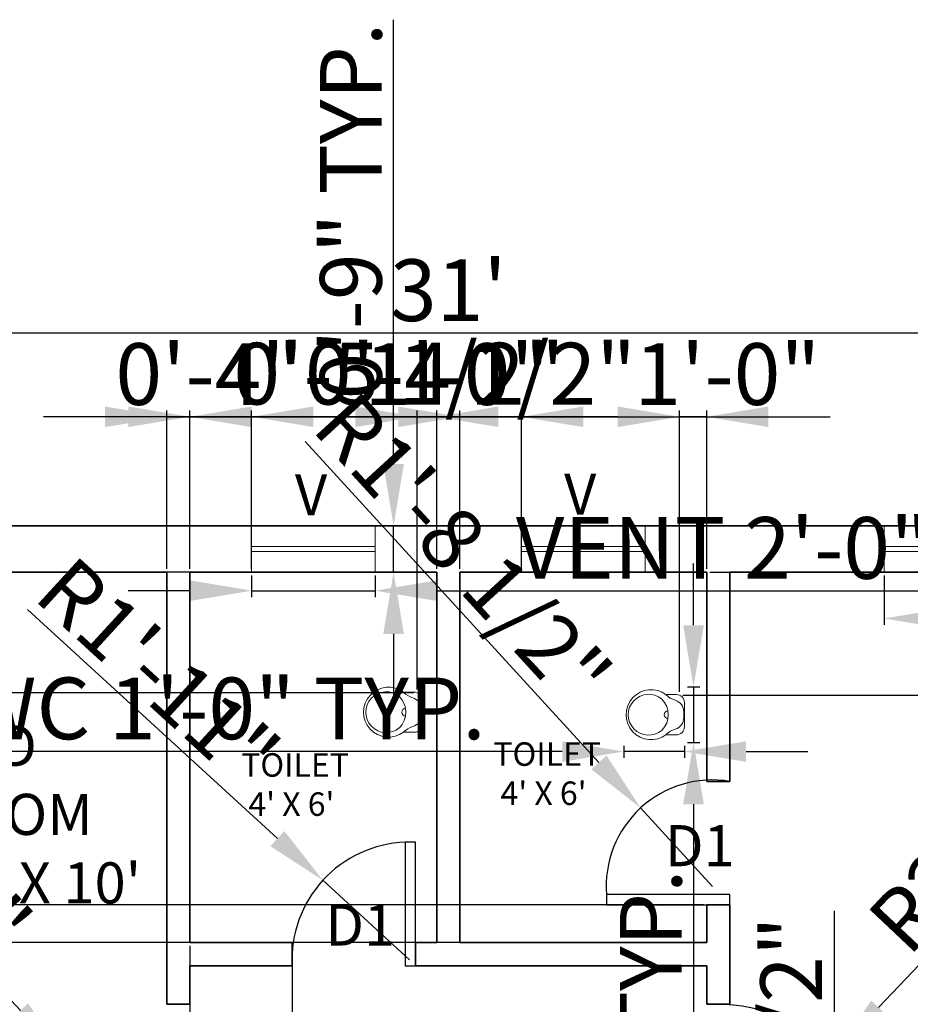
# Model space of a CAD drawing. Units: inches. Extents: x 2122 to 2726, y 1923 to 2370.
# Tile 4 of 6: x 2333 to 2506, y 2178 to 2370. Entities that reach past the tile are written whole.
import ezdxf

# ---------------------------------------------------------------- set-up
doc = ezdxf.new("R2010")
doc.units = ezdxf.units.IN
for name, color, linetype, lineweight in [('A-ANNO-DIMS', 2, 'Continuous', 18), ('A-ANNO-TEXT', 7, 'Continuous', 18), ('A-AREA-IDEN', 7, 'Continuous', 25), ('A-DOOR', 3, 'Continuous', 25), ('A-FLOR-FIXT', 9, 'Continuous', 18), ('A-GLAZ', 4, 'Continuous', 18), ('A-WALL', 7, 'Continuous', 35)]:
    doc.layers.add(name, color=color, linetype=linetype, lineweight=lineweight)
doc.styles.get("Standard").update_dxf_attribs({"font": 'arial.ttf'})
doc.dimstyles.new('ISO-25', dxfattribs={"dimtxt": 12, "dimasz": 12, "dimexe": 1.25, "dimexo": 0.625, "dimtad": 1, "dimlunit": 3, "dimtxsty": 'Standard', "dimcen": 2.5, "dimadec": 0, "dimazin": 0, "dimtfac": 1, "dimtmove": 0, "dimatfit": 3, "dimfxl": 1, "dimarcsym": 0})

# ---------------------------------------------------------------- blocks, each defined once
blk = doc.blocks.new('A$C6EF51710')
at = {"linetype": 'ByBlock'}
for p, q in [((0.0508, 0.2843), (0.1169, 0.2843)), ((0, 0.0811), (0, 0.2335)), ((0.0041, 0.1392), (0.0041, 0.1755)), ((0.1169, 0.0303), (0.0508, 0.0303))]:
    blk.add_line(p, q, dxfattribs=at)
for centre, radius, start, end in [((0.2107, 0.1573), 0.1576, 232.89836, 127.10164), ((0.0508, 0.2335), 0.0508, 90, 180), ((0.0168, 0.3818), 0.1397, 287.10464, 315), ((0.2413, 0.1573), 0.1397, 135, 225), ((0.2254, 0.1573), 0.1289, 230.00836, 129.99164), ((0.0803, 0.1755), 0.0762, 107.10464, 180), ((0.0803, 0.1392), 0.0762, 180, 252.89536), ((0.1016, 0.1573), 0.0254, 275.21591, 84.78409), ((0.0508, 0.0811), 0.0508, 180, 270), ((0.0168, -0.0672), 0.1397, 45, 72.89536)]:
    blk.add_arc(centre, radius, start, end, dxfattribs=at)
blk = doc.blocks.new('*D10')
at = {"layer": 'A-ANNO-DIMS', "color": 0, "lineweight": -2, "transparency": 16777216}
for p, q in [((2232.51, 2271.86), (2232.51, 2309.99)), ((2244.51, 2308.74), (2588.01, 2308.74)), ((2600.01, 2271.86), (2600.01, 2309.99))]:
    blk.add_line(p, q, dxfattribs=at)
at = {"layer": 'A-ANNO-DIMS', "color": 0, "transparency": 16777216}
for points in [[(2244.51, 2310.74), (2244.51, 2306.74), (2232.51, 2308.74)], [(2588.01, 2310.74), (2588.01, 2306.74), (2600.01, 2308.74)]]:
    blk.add_solid(points, dxfattribs=at)
at = {"layer": 'Defpoints', "color": 0, "transparency": 16777216}
for p in [(2600.01, 2308.74), (2232.51, 2271.24), (2600.01, 2271.24)]:
    blk.add_point(p, dxfattribs=at)
at = {"layer": 'A-ANNO-DIMS', "color": 0, "transparency": 16777216, "insert": (2416.26, 2315.49), "char_height": 12, "attachment_point": 5}
blk.add_mtext("31'", dxfattribs=at)
blk = doc.blocks.new('WIN-60IN')
for p, q in [((0, 0), (0, 9)), ((60, 0), (60, 9)), ((0, 5), (60, 5)), ((0, 4), (60, 4))]:
    blk.add_line(p, q)
blk = doc.blocks.new('VENT-24IN')
for p, q in [((0, 0), (0, 9)), ((24, 0), (24, 9)), ((0, 5), (24, 5)), ((0, 4), (24, 4))]:
    blk.add_line(p, q)
blk = doc.blocks.new('DOOR-LEAF-24IN')
for p, q in [((2, 24), (0, 24)), ((0, 24), (0, 0)), ((2, 0), (2, 24)), ((0, 0), (2, 0))]:
    blk.add_line(p, q)
blk = doc.blocks.new('*D16')
at = {"layer": 'A-ANNO-DIMS', "color": 0, "lineweight": -2, "transparency": 16777216}
for p, q in [((2501.01, 2261.61), (2501.01, 2251.99)), ((2561.01, 2261.61), (2561.01, 2251.99)), ((2513.01, 2253.24), (2549.01, 2253.24)), ((2561.01, 2253.24), (2726.11, 2253.24))]:
    blk.add_line(p, q, dxfattribs=at)
at = {"layer": 'A-ANNO-DIMS', "color": 0, "transparency": 16777216}
for points in [[(2513.01, 2255.24), (2513.01, 2251.24), (2501.01, 2253.24)], [(2549.01, 2255.24), (2549.01, 2251.24), (2561.01, 2253.24)]]:
    blk.add_solid(points, dxfattribs=at)
at = {"layer": 'Defpoints', "color": 0, "transparency": 16777216}
for p in [(2501.01, 2262.24), (2561.01, 2262.24), (2561.01, 2253.24)]:
    blk.add_point(p, dxfattribs=at)
at = {"layer": 'A-ANNO-DIMS', "color": 0, "transparency": 16777216, "insert": (2649.56, 2260.07), "char_height": 12, "attachment_point": 5}
blk.add_mtext('WINDOW 5\'-0" TYP.', dxfattribs=at)
blk = doc.blocks.new('*D20')
at = {"layer": 'A-ANNO-DIMS', "color": 0, "lineweight": -2, "transparency": 16777216}
for p, q in [((2378.01, 2261.61), (2378.01, 2257.39)), ((2402.01, 2261.61), (2402.01, 2257.39)), ((2366.01, 2258.64), (2354.01, 2258.64)), ((2378.01, 2258.64), (2402.01, 2258.64)), ((2414.01, 2258.64), (2550.39, 2258.64))]:
    blk.add_line(p, q, dxfattribs=at)
at = {"layer": 'A-ANNO-DIMS', "color": 0, "transparency": 16777216}
for points in [[(2366.01, 2260.64), (2366.01, 2256.64), (2378.01, 2258.64)], [(2414.01, 2260.64), (2414.01, 2256.64), (2402.01, 2258.64)]]:
    blk.add_solid(points, dxfattribs=at)
at = {"layer": 'Defpoints', "color": 0, "transparency": 16777216}
for p in [(2378.01, 2262.24), (2402.01, 2262.24), (2402.01, 2258.64)]:
    blk.add_point(p, dxfattribs=at)
at = {"layer": 'A-ANNO-DIMS', "color": 0, "transparency": 16777216, "insert": (2488.2, 2265.39), "char_height": 12, "attachment_point": 5}
blk.add_mtext('VENT 2\'-0" TYP.', dxfattribs=at)
blk = doc.blocks.new('*D21')
at = {"layer": 'A-ANNO-DIMS', "color": 0, "lineweight": -2, "transparency": 16777216}
for p, q in [((2405.61, 2283.24), (2405.61, 2369.63)), ((2402.63, 2271.24), (2406.86, 2271.24)), ((2405.61, 2262.24), (2405.61, 2271.24)), ((2402.63, 2262.24), (2406.86, 2262.24)), ((2405.61, 2250.24), (2405.61, 2238.24))]:
    blk.add_line(p, q, dxfattribs=at)
at = {"layer": 'A-ANNO-DIMS', "color": 0, "transparency": 16777216}
for points in [[(2403.61, 2283.24), (2407.61, 2283.24), (2405.61, 2271.24)], [(2403.61, 2250.24), (2407.61, 2250.24), (2405.61, 2262.24)]]:
    blk.add_solid(points, dxfattribs=at)
at = {"layer": 'Defpoints', "color": 0, "transparency": 16777216}
for p in [(2402.01, 2271.24), (2405.61, 2271.24), (2402.01, 2262.24)]:
    blk.add_point(p, dxfattribs=at)
at = {"layer": 'A-ANNO-DIMS', "color": 0, "transparency": 16777216, "insert": (2398.86, 2332.43), "char_height": 12, "attachment_point": 5, "rotation": 90}
blk.add_mtext('0\'-9" TYP.', dxfattribs=at)
blk = doc.blocks.new('*D22')
at = {"layer": 'A-ANNO-DIMS', "color": 0, "lineweight": -2, "transparency": 16777216}
for p, q in [((2330.01, 2149.64), (2142.68, 2149.64)), ((2330.01, 2144.86), (2330.01, 2150.89)), ((2354.01, 2149.64), (2342.01, 2149.64)), ((2366.01, 2144.86), (2366.01, 2150.89))]:
    blk.add_line(p, q, dxfattribs=at)
at = {"layer": 'A-ANNO-DIMS', "color": 0, "transparency": 16777216}
for points in [[(2342.01, 2151.64), (2342.01, 2147.64), (2330.01, 2149.64)], [(2354.01, 2151.64), (2354.01, 2147.64), (2366.01, 2149.64)]]:
    blk.add_solid(points, dxfattribs=at)
at = {"layer": 'Defpoints', "color": 0, "transparency": 16777216}
for p in [(2330.01, 2149.64), (2330.01, 2144.24), (2366.01, 2144.24)]:
    blk.add_point(p, dxfattribs=at)
at = {"layer": 'A-ANNO-DIMS', "color": 0, "transparency": 16777216, "insert": (2230.34, 2156.47), "char_height": 12, "attachment_point": 5}
blk.add_mtext('DOOR LEAF 3\'-0" TYP.', dxfattribs=at)
blk = doc.blocks.new('*D28')
at = {"layer": 'A-ANNO-DIMS', "color": 0, "lineweight": -2, "transparency": 16777216}
for p, q in [((2450.4, 2228.51), (2450.4, 2226.12)), ((2462.17, 2228.51), (2462.17, 2226.12)), ((2438.4, 2227.37), (2318.92, 2227.37)), ((2462.17, 2227.37), (2450.4, 2227.37)), ((2474.17, 2227.37), (2486.17, 2227.37))]:
    blk.add_line(p, q, dxfattribs=at)
at = {"layer": 'A-ANNO-DIMS', "color": 0, "transparency": 16777216}
for points in [[(2438.4, 2229.37), (2438.4, 2225.37), (2450.4, 2227.37)], [(2474.17, 2229.37), (2474.17, 2225.37), (2462.17, 2227.37)]]:
    blk.add_solid(points, dxfattribs=at)
at = {"layer": 'Defpoints', "color": 0, "transparency": 16777216}
for p in [(2450.4, 2229.14), (2462.17, 2229.14), (2450.4, 2227.37)]:
    blk.add_point(p, dxfattribs=at)
at = {"layer": 'A-ANNO-DIMS', "color": 0, "transparency": 16777216, "insert": (2372.66, 2234.2), "char_height": 12, "attachment_point": 5}
blk.add_mtext('WC 1\'-0" TYP.', dxfattribs=at)
blk = doc.blocks.new('*D29')
at = {"layer": 'A-ANNO-DIMS', "color": 0, "lineweight": -2, "transparency": 16777216}
for p, q in [((2463.94, 2251.92), (2463.94, 2263.92)), ((2462.8, 2239.92), (2465.19, 2239.92)), ((2463.94, 2239.92), (2463.94, 2229.14)), ((2462.8, 2229.14), (2465.19, 2229.14)), ((2463.94, 2217.14), (2463.94, 2121.42))]:
    blk.add_line(p, q, dxfattribs=at)
at = {"layer": 'A-ANNO-DIMS', "color": 0, "transparency": 16777216}
for points in [[(2461.94, 2251.92), (2465.94, 2251.92), (2463.94, 2239.92)], [(2461.94, 2217.14), (2465.94, 2217.14), (2463.94, 2229.14)]]:
    blk.add_solid(points, dxfattribs=at)
at = {"layer": 'Defpoints', "color": 0, "transparency": 16777216}
for p in [(2462.17, 2239.92), (2462.17, 2229.14), (2463.94, 2229.14)]:
    blk.add_point(p, dxfattribs=at)
at = {"layer": 'A-ANNO-DIMS', "color": 0, "transparency": 16777216, "insert": (2457.19, 2163.28), "char_height": 12, "attachment_point": 5, "rotation": 90}
blk.add_mtext('0\'-11" TYP.', dxfattribs=at)
blk = doc.blocks.new('*D36')
at = {"layer": 'A-ANNO-DIMS', "color": 0, "lineweight": -2, "transparency": 16777216}
for p, q in [((2491.33, 2053.12), (2491.33, 2196.38)), ((2482.88, 2053.12), (2492.58, 2053.12)), ((2491.33, 2004.66), (2491.33, 2041.12)), ((2482.88, 1992.66), (2492.58, 1992.66))]:
    blk.add_line(p, q, dxfattribs=at)
at = {"layer": 'A-ANNO-DIMS', "color": 0, "transparency": 16777216}
for points in [[(2489.33, 2041.12), (2493.33, 2041.12), (2491.33, 2053.12)], [(2489.33, 2004.66), (2493.33, 2004.66), (2491.33, 1992.66)]]:
    blk.add_solid(points, dxfattribs=at)
at = {"layer": 'Defpoints', "color": 0, "transparency": 16777216}
for p in [(2482.26, 2053.12), (2491.33, 2053.12), (2482.26, 1992.66)]:
    blk.add_point(p, dxfattribs=at)
at = {"layer": 'A-ANNO-DIMS', "color": 0, "transparency": 16777216, "insert": (2484.5, 2130.75), "char_height": 12, "attachment_point": 5, "rotation": 90}
blk.add_mtext('TV UNIT 5\'-0 1/2"', dxfattribs=at)
blk = doc.blocks.new('*D39')
at = {"layer": 'A-ANNO-DIMS', "color": 0, "lineweight": -2, "transparency": 16777216}
for p, q in [((2361.51, 2262.86), (2361.51, 2293.69)), ((2366.01, 2262.86), (2366.01, 2293.69)), ((2349.51, 2292.44), (2337.51, 2292.44)), ((2361.51, 2292.44), (2366.01, 2292.44)), ((2378.01, 2292.44), (2451.12, 2292.44))]:
    blk.add_line(p, q, dxfattribs=at)
at = {"layer": 'A-ANNO-DIMS', "color": 0, "transparency": 16777216}
for points in [[(2349.51, 2294.44), (2349.51, 2290.44), (2361.51, 2292.44)], [(2378.01, 2294.44), (2378.01, 2290.44), (2366.01, 2292.44)]]:
    blk.add_solid(points, dxfattribs=at)
at = {"layer": 'Defpoints', "color": 0, "transparency": 16777216}
for p in [(2366.01, 2292.44), (2361.51, 2262.24), (2366.01, 2262.24)]:
    blk.add_point(p, dxfattribs=at)
at = {"layer": 'A-ANNO-DIMS', "color": 0, "transparency": 16777216, "insert": (2420.56, 2299.27), "char_height": 12, "attachment_point": 5}
blk.add_mtext('0\'-4 1/2"', dxfattribs=at)
blk = doc.blocks.new('*D43')
at = {"layer": 'A-ANNO-DIMS', "color": 0, "lineweight": -2, "transparency": 16777216}
for p, q in [((2366.01, 2262.86), (2366.01, 2293.69)), ((2378.01, 2262.86), (2378.01, 2293.69)), ((2354.01, 2292.44), (2342.01, 2292.44)), ((2366.01, 2292.44), (2378.01, 2292.44)), ((2390.01, 2292.44), (2434.03, 2292.44))]:
    blk.add_line(p, q, dxfattribs=at)
at = {"layer": 'A-ANNO-DIMS', "color": 0, "transparency": 16777216}
for points in [[(2354.01, 2294.44), (2354.01, 2290.44), (2366.01, 2292.44)], [(2390.01, 2294.44), (2390.01, 2290.44), (2378.01, 2292.44)]]:
    blk.add_solid(points, dxfattribs=at)
at = {"layer": 'Defpoints', "color": 0, "transparency": 16777216}
for p in [(2378.01, 2292.44), (2366.01, 2262.24), (2378.01, 2262.24)]:
    blk.add_point(p, dxfattribs=at)
at = {"layer": 'A-ANNO-DIMS', "color": 0, "transparency": 16777216, "insert": (2418.02, 2299.19), "char_height": 12, "attachment_point": 5}
blk.add_mtext('1\'-0"', dxfattribs=at)
blk = doc.blocks.new('*D44')
at = {"layer": 'A-ANNO-DIMS', "color": 0, "lineweight": -2, "transparency": 16777216}
for p, q in [((2418.51, 2262.86), (2418.51, 2293.69)), ((2430.51, 2262.86), (2430.51, 2293.69)), ((2406.51, 2292.44), (2394.51, 2292.44)), ((2418.51, 2292.44), (2430.51, 2292.44)), ((2442.51, 2292.44), (2486.53, 2292.44))]:
    blk.add_line(p, q, dxfattribs=at)
at = {"layer": 'A-ANNO-DIMS', "color": 0, "transparency": 16777216}
for points in [[(2406.51, 2294.44), (2406.51, 2290.44), (2418.51, 2292.44)], [(2442.51, 2294.44), (2442.51, 2290.44), (2430.51, 2292.44)]]:
    blk.add_solid(points, dxfattribs=at)
at = {"layer": 'Defpoints', "color": 0, "transparency": 16777216}
for p in [(2430.51, 2292.44), (2418.51, 2262.24), (2430.51, 2262.24)]:
    blk.add_point(p, dxfattribs=at)
at = {"layer": 'A-ANNO-DIMS', "color": 0, "transparency": 16777216, "insert": (2470.52, 2299.19), "char_height": 12, "attachment_point": 5}
blk.add_mtext('1\'-0"', dxfattribs=at)
blk = doc.blocks.new('*D50')
at = {"layer": 'A-ANNO-DIMS', "color": 0, "lineweight": -2, "transparency": 16777216}
for p, q in [((2366.01, 2189.61), (2366.01, 1950.29)), ((2385.88, 2189.61), (2385.88, 1950.29)), ((2354.01, 1951.54), (2342.01, 1951.54)), ((2366.01, 1951.54), (2385.88, 1951.54)), ((2397.88, 1951.54), (2441.9, 1951.54))]:
    blk.add_line(p, q, dxfattribs=at)
at = {"layer": 'A-ANNO-DIMS', "color": 0, "transparency": 16777216}
for points in [[(2354.01, 1953.54), (2354.01, 1949.54), (2366.01, 1951.54)], [(2397.88, 1953.54), (2397.88, 1949.54), (2385.88, 1951.54)]]:
    blk.add_solid(points, dxfattribs=at)
at = {"layer": 'Defpoints', "color": 0, "transparency": 16777216}
for p in [(2366.01, 2190.24), (2385.88, 2190.24), (2385.88, 1951.54)]:
    blk.add_point(p, dxfattribs=at)
at = {"layer": 'A-ANNO-DIMS', "color": 0, "transparency": 16777216, "insert": (2425.89, 1958.29), "char_height": 12, "attachment_point": 5}
blk.add_mtext('1\'-8"', dxfattribs=at)
blk = doc.blocks.new('*D51')
at = {"layer": 'A-ANNO-DIMS', "color": 0, "lineweight": -2, "transparency": 16777216}
for p, q in [((2211.31, 2209.57), (2211.31, 2282.68)), ((2465.88, 2197.57), (2210.06, 2197.57)), ((2211.31, 2190.24), (2211.31, 2197.57)), ((2465.88, 2190.24), (2210.06, 2190.24)), ((2211.31, 2178.24), (2211.31, 2166.24))]:
    blk.add_line(p, q, dxfattribs=at)
at = {"layer": 'A-ANNO-DIMS', "color": 0, "transparency": 16777216}
for points in [[(2209.31, 2209.57), (2213.31, 2209.57), (2211.31, 2197.57)], [(2209.31, 2178.24), (2213.31, 2178.24), (2211.31, 2190.24)]]:
    blk.add_solid(points, dxfattribs=at)
at = {"layer": 'Defpoints', "color": 0, "transparency": 16777216}
for p in [(2211.31, 2197.57), (2466.51, 2197.57), (2466.51, 2190.24)]:
    blk.add_point(p, dxfattribs=at)
at = {"layer": 'A-ANNO-DIMS', "color": 0, "transparency": 16777216, "insert": (2204.48, 2252.12), "char_height": 12, "attachment_point": 5, "rotation": 90}
blk.add_mtext('0\'-7 1/2"', dxfattribs=at)
blk = doc.blocks.new('*D64')
at = {"layer": 'A-ANNO-DIMS', "color": 0, "lineweight": -2, "transparency": 16777216}
for p, q in [((2410.17, 2239.43), (2410.17, 2293.69)), ((2414.01, 2262.86), (2414.01, 2293.69)), ((2398.17, 2292.44), (2353.02, 2292.44)), ((2414.01, 2292.44), (2410.17, 2292.44)), ((2426.01, 2292.44), (2438.01, 2292.44))]:
    blk.add_line(p, q, dxfattribs=at)
at = {"layer": 'A-ANNO-DIMS', "color": 0, "transparency": 16777216}
for points in [[(2398.17, 2294.44), (2398.17, 2290.44), (2410.17, 2292.44)], [(2426.01, 2294.44), (2426.01, 2290.44), (2414.01, 2292.44)]]:
    blk.add_solid(points, dxfattribs=at)
at = {"layer": 'Defpoints', "color": 0, "transparency": 16777216}
for p in [(2410.17, 2292.44), (2414.01, 2262.24), (2410.17, 2238.81)]:
    blk.add_point(p, dxfattribs=at)
at = {"layer": 'A-ANNO-DIMS', "color": 0, "transparency": 16777216, "insert": (2369.59, 2299.19), "char_height": 12, "attachment_point": 5}
blk.add_mtext('0\'-4"', dxfattribs=at)
blk = doc.blocks.new('*D65')
at = {"layer": 'A-ANNO-DIMS', "color": 0, "lineweight": -2, "transparency": 16777216}
for p, q in [((2211.31, 2274.24), (2211.31, 2286.24)), ((2413.38, 2262.24), (2210.06, 2262.24)), ((2211.31, 2262.24), (2211.31, 2238.81)), ((2409.54, 2238.81), (2210.06, 2238.81)), ((2211.31, 2226.81), (2211.31, 2145.5))]:
    blk.add_line(p, q, dxfattribs=at)
at = {"layer": 'A-ANNO-DIMS', "color": 0, "transparency": 16777216}
for points in [[(2209.31, 2274.24), (2213.31, 2274.24), (2211.31, 2262.24)], [(2209.31, 2226.81), (2213.31, 2226.81), (2211.31, 2238.81)]]:
    blk.add_solid(points, dxfattribs=at)
at = {"layer": 'Defpoints', "color": 0, "transparency": 16777216}
for p in [(2414.01, 2262.24), (2211.31, 2238.81), (2410.17, 2238.81)]:
    blk.add_point(p, dxfattribs=at)
at = {"layer": 'A-ANNO-DIMS', "color": 0, "transparency": 16777216, "insert": (2204.48, 2180.16), "char_height": 12, "attachment_point": 5, "rotation": 90}
blk.add_mtext('1\'-11 1/2"', dxfattribs=at)
blk = doc.blocks.new('*D66')
at = {"layer": 'A-ANNO-DIMS', "color": 0, "lineweight": -2, "transparency": 16777216}
for p, q in [((2461.22, 2238.95), (2461.22, 2293.69)), ((2466.51, 2262.86), (2466.51, 2293.69)), ((2449.22, 2292.44), (2376.1, 2292.44)), ((2466.51, 2292.44), (2461.22, 2292.44)), ((2478.51, 2292.44), (2490.51, 2292.44))]:
    blk.add_line(p, q, dxfattribs=at)
at = {"layer": 'A-ANNO-DIMS', "color": 0, "transparency": 16777216}
for points in [[(2449.22, 2294.44), (2449.22, 2290.44), (2461.22, 2292.44)], [(2478.51, 2294.44), (2478.51, 2290.44), (2466.51, 2292.44)]]:
    blk.add_solid(points, dxfattribs=at)
at = {"layer": 'Defpoints', "color": 0, "transparency": 16777216}
for p in [(2461.22, 2292.44), (2466.51, 2262.24), (2461.22, 2238.32)]:
    blk.add_point(p, dxfattribs=at)
at = {"layer": 'A-ANNO-DIMS', "color": 0, "transparency": 16777216, "insert": (2406.66, 2299.27), "char_height": 12, "attachment_point": 5}
blk.add_mtext('0\'-5 1/2"', dxfattribs=at)
blk = doc.blocks.new('*D67')
at = {"layer": 'A-ANNO-DIMS', "color": 0, "lineweight": -2, "transparency": 16777216}
for p, q in [((2621.21, 2274.24), (2621.21, 2286.24)), ((2467.13, 2262.24), (2622.46, 2262.24)), ((2621.21, 2262.24), (2621.21, 2238.32)), ((2461.84, 2238.32), (2622.46, 2238.32)), ((2621.21, 2226.32), (2621.21, 2180.97))]:
    blk.add_line(p, q, dxfattribs=at)
at = {"layer": 'A-ANNO-DIMS', "color": 0, "transparency": 16777216}
for points in [[(2619.21, 2274.24), (2623.21, 2274.24), (2621.21, 2262.24)], [(2619.21, 2226.32), (2623.21, 2226.32), (2621.21, 2238.32)]]:
    blk.add_solid(points, dxfattribs=at)
at = {"layer": 'Defpoints', "color": 0, "transparency": 16777216}
for p in [(2466.51, 2262.24), (2461.22, 2238.32), (2621.21, 2238.32)]:
    blk.add_point(p, dxfattribs=at)
at = {"layer": 'A-ANNO-DIMS', "color": 0, "transparency": 16777216, "insert": (2614.46, 2197.64), "char_height": 12, "attachment_point": 5, "rotation": 90}
blk.add_mtext('2\'-0"', dxfattribs=at)
blk = doc.blocks.new('*D70')
at = {"layer": 'A-ANNO-DIMS', "color": 0, "lineweight": -2, "transparency": 16777216}
for p, q in [((2274.99, 2238.55), (2333.07, 2177.05)), ((2366.24, 2141.93), (2341.31, 2168.33))]:
    blk.add_line(p, q, dxfattribs=at)
at = {"layer": 'A-ANNO-DIMS', "color": 0, "transparency": 16777216}
blk.add_solid([(2334.53, 2178.42), (2331.62, 2175.68), (2341.31, 2168.33)], dxfattribs=at)
at = {"layer": 'Defpoints', "color": 0, "transparency": 16777216}
for p in [(2341.31, 2168.33), (2366.24, 2141.93)]:
    blk.add_point(p, dxfattribs=at)
at = {"layer": 'A-ANNO-DIMS', "color": 0, "transparency": 16777216, "insert": (2304.88, 2216.85), "char_height": 12, "attachment_point": 5, "rotation": 313.3629}
blk.add_mtext('R3\'-0 1/2"', dxfattribs=at)
blk = doc.blocks.new('*D71')
at = {"layer": 'A-ANNO-DIMS', "color": 0, "lineweight": -2, "transparency": 16777216}
for p, q in [((2564.44, 2245.87), (2499.95, 2177.59)), ((2468.06, 2143.82), (2491.71, 2168.87))]:
    blk.add_line(p, q, dxfattribs=at)
at = {"layer": 'A-ANNO-DIMS', "color": 0, "transparency": 16777216}
blk.add_solid([(2498.5, 2178.96), (2501.41, 2176.22), (2491.71, 2168.87)], dxfattribs=at)
at = {"layer": 'Defpoints', "color": 0, "transparency": 16777216}
for p in [(2491.71, 2168.87), (2468.06, 2143.82)]:
    blk.add_point(p, dxfattribs=at)
at = {"layer": 'A-ANNO-DIMS', "color": 0, "transparency": 16777216, "insert": (2531.35, 2220.78), "char_height": 12, "attachment_point": 5, "rotation": 46.6362}
blk.add_mtext('R2\'-10 1/2"', dxfattribs=at)
blk = doc.blocks.new('*D74')
at = {"layer": 'A-ANNO-DIMS', "color": 0, "lineweight": -2, "transparency": 16777216}
for p, q in [((2334.39, 2255.01), (2383.01, 2210.44)), ((2408.72, 2186.88), (2391.86, 2202.34))]:
    blk.add_line(p, q, dxfattribs=at)
at = {"layer": 'A-ANNO-DIMS', "color": 0, "transparency": 16777216}
blk.add_solid([(2384.36, 2211.92), (2381.66, 2208.97), (2391.86, 2202.34)], dxfattribs=at)
at = {"layer": 'Defpoints', "color": 0, "transparency": 16777216}
for p in [(2391.86, 2202.34), (2408.72, 2186.88)]:
    blk.add_point(p, dxfattribs=at)
at = {"layer": 'A-ANNO-DIMS', "color": 0, "transparency": 16777216, "insert": (2358.77, 2241.68), "char_height": 12, "attachment_point": 5, "rotation": 317.4903}
blk.add_mtext('R1\'-11"', dxfattribs=at)
blk = doc.blocks.new('*D75')
at = {"layer": 'A-ANNO-DIMS', "color": 0, "lineweight": -2, "transparency": 16777216}
for p, q in [((2388.39, 2287.61), (2445.55, 2225.25)), ((2467.65, 2201.14), (2453.66, 2216.4))]:
    blk.add_line(p, q, dxfattribs=at)
at = {"layer": 'A-ANNO-DIMS', "color": 0, "transparency": 16777216}
blk.add_solid([(2447.03, 2226.6), (2444.08, 2223.9), (2453.66, 2216.4)], dxfattribs=at)
at = {"layer": 'Defpoints', "color": 0, "transparency": 16777216}
for p in [(2453.66, 2216.4), (2467.65, 2201.14)]:
    blk.add_point(p, dxfattribs=at)
at = {"layer": 'A-ANNO-DIMS', "color": 0, "transparency": 16777216, "insert": (2417.95, 2265.46), "char_height": 12, "attachment_point": 5, "rotation": 312.5118}
blk.add_mtext('R1\'-8 1/2"', dxfattribs=at)

msp = doc.modelspace()

# ---------------------------------------------------------------- linework, layer by layer
at = {"layer": 'A-DOOR'}
for centre, radius, start, end in [((2467.648, 2201.143), 20.7, 80.65968, 184.36121), ((2408.715, 2186.884), 22.868, 92.10212, 182.87699), ((2468.058, 2143.819), 34.452, 0.69324, 92.57991)]:
    msp.add_arc(centre, radius, start, end, dxfattribs=at)
at = {"layer": 'A-WALL'}
for p, q in [((2232.508, 2271.236), (2600.008, 2271.236)), ((2241.508, 2262.236), (2361.508, 2262.236)), ((2361.508, 2178.236), (2361.508, 2262.236)), ((2366.008, 2262.236), (2414.008, 2262.236)), ((2366.008, 2190.236), (2366.008, 2262.236)), ((2414.008, 2190.236), (2414.008, 2262.236)), ((2418.508, 2190.236), (2418.508, 2262.236)), ((2418.508, 2262.236), (2466.508, 2262.236)), ((2466.508, 2221.569), (2466.508, 2262.236)), ((2471.008, 2262.236), (2591.008, 2262.236)), ((2471.008, 2221.569), (2471.008, 2262.236)), ((2466.508, 2221.569), (2471.008, 2221.569)), ((2466.508, 2190.236), (2466.508, 2197.569)), ((2466.508, 2197.569), (2471.008, 2197.569)), ((2471.008, 2178.236), (2471.008, 2197.569)), ((2366.008, 2190.236), (2385.877, 2190.236)), ((2385.877, 2190.236), (2385.877, 2185.736)), ((2409.877, 2190.236), (2409.877, 2185.736)), ((2409.877, 2190.236), (2414.008, 2190.236)), ((2418.508, 2190.236), (2466.508, 2190.236)), ((2366.008, 2185.736), (2385.877, 2185.736)), ((2366.008, 2178.236), (2366.008, 2185.736)), ((2409.877, 2185.736), (2418.508, 2185.736)), ((2418.508, 2185.736), (2466.508, 2185.736)), ((2466.508, 2178.236), (2466.508, 2185.736)), ((2361.508, 2178.236), (2366.008, 2178.236)), ((2471.008, 2178.236), (2466.508, 2178.236))]:
    msp.add_line(p, q, dxfattribs=at)

# ---------------------------------------------------------------- block references
at = {"layer": 'A-DOOR'}
msp.add_blockref('DOOR-LEAF-24IN', (2407.877, 2185.736), dxfattribs=at)
at = {"layer": 'A-DOOR', "rotation": 270.0000000000043}
msp.add_blockref('DOOR-LEAF-24IN', (2447.008, 2199.569), dxfattribs=at)
at = {"layer": 'A-FLOR-FIXT', "xscale": 30.82221554952108, "yscale": 30.82221554952108, "zscale": 30.82221554952108, "rotation": 180}
for p in [(2411.123, 2239.867), (2462.172, 2239.379)]:
    msp.add_blockref('A$C6EF51710', p, dxfattribs=at)
at = {"layer": 'A-GLAZ'}
for name, p in [('VENT-24IN', (2378.008, 2262.236)), ('VENT-24IN', (2430.508, 2262.236)), ('WIN-60IN', (2501.008, 2262.236))]:
    msp.add_blockref(name, p, dxfattribs=at)

# ---------------------------------------------------------------- texts
at = {"layer": 'A-ANNO-TEXT', "attachment_point": 1}
for s, insert, char_height in [('V', (2386.426, 2281.247), 7.99), ('V', (2438.772, 2281.399), 7.99), ('D1', (2458.399, 2213.067), 7.9897), ('D1', (2392.36, 2197.646), 7.9897)]:
    msp.add_mtext_dynamic_manual_height_columns(s, width=65.06795, gutter_width=39.949, heights=[0], dxfattribs=dict(at, insert=insert, char_height=char_height))
at = {"layer": 'A-AREA-IDEN', "attachment_point": 1}
for s, width, gutter_width, insert, char_height in [("BED\\PROOM \\P10' X 10'", 65.06795, 39.949, (2315.153, 2232.468), 7.9897), ("   TOILET \\P    4' X 6'", 37.18666, 22.831, (2420.826, 2229.161), 4.56616), ("   TOILET \\P    4' X 6'", 37.18666, 22.831, (2371.791, 2227.046), 4.56616)]:
    msp.add_mtext_dynamic_manual_height_columns(s, width=width, gutter_width=gutter_width, heights=[0], dxfattribs=dict(at, insert=insert, char_height=char_height))

# ---------------------------------------------------------------- dimensions: what is measured, and where the dimension line sits
at = {"layer": 'A-ANNO-DIMS'}
for base, p1, p2, angle, text, picture, middle in [((2405.608, 2271.236), (2402.008, 2262.236), (2402.008, 2271.236), 90, '<> TYP.', '*D21', (2398.856, 2332.434)), ((2463.938, 2229.14), (2462.172, 2239.919), (2462.172, 2229.14), 270, '<> TYP.', '*D29', (2457.186, 2163.28)), ((2450.397, 2227.374), (2462.172, 2229.14), (2450.397, 2229.14), 180, 'WC <> TYP.', '*D28', (2372.66, 2234.203)), ((2491.325, 2053.118), (2482.256, 1992.656), (2482.256, 2053.118), 90, 'TV UNIT <>', '*D36', (2484.496, 2130.749)), ((2330.008, 2149.636), (2366.008, 2144.236), (2330.008, 2144.236), 180, 'DOOR LEAF <> TYP.', '*D22', (2230.342, 2156.474))]:
    dim = msp.add_linear_dim(base=base, p1=p1, p2=p2, angle=angle, text=text, dimstyle='ISO-25', override={"dimdec": 1, "dimlfac": 1, "dimrnd": 0, "dimzin": 1, "dimdsep": 46, "dimlunit": 4, "dimfrac": 2}, dxfattribs=at)
    dim.commit()
    dim.dimension.update_dxf_attribs({"geometry": picture, "text_midpoint": middle})
for base, p1, p2, text, override, picture, middle in [((2600.008, 2308.735), (2232.508, 2271.236), (2600.008, 2271.236), "31'", {"dimclrd": 0, "dimclre": 0, "dimclrt": 0}, '*D10', (2416.258, 2315.491)), ((2402.008, 2258.636), (2378.008, 2262.236), (2402.008, 2262.236), 'VENT <> TYP.', {"dimdec": 1, "dimlfac": 1, "dimrnd": 0, "dimzin": 1, "dimdsep": 46, "dimlunit": 4, "dimfrac": 2}, '*D20', (2488.2, 2265.388)), ((2561.008, 2253.236), (2501.008, 2262.236), (2561.008, 2262.236), 'WINDOW <> TYP.', {"dimdec": 1, "dimlfac": 1, "dimrnd": 0, "dimzin": 1, "dimdsep": 46, "dimlunit": 4, "dimfrac": 2}, '*D16', (2649.558, 2260.07))]:
    dim = msp.add_linear_dim(base=base, p1=p1, p2=p2, text=text, dimstyle='ISO-25', override=override, dxfattribs=at)
    dim.commit()
    dim.dimension.update_dxf_attribs({"geometry": picture, "text_midpoint": middle})
for base, p1, p2, picture, middle in [((2366.008, 2292.436), (2361.508, 2262.236), (2366.008, 2262.236), '*D39', (2420.563, 2299.266)), ((2461.216, 2292.436), (2466.508, 2262.236), (2461.216, 2238.321), '*D66', (2406.66, 2299.266)), ((2378.008, 2292.436), (2366.008, 2262.236), (2378.008, 2262.236), '*D43', (2418.017, 2299.188)), ((2410.167, 2292.436), (2414.008, 2262.236), (2410.167, 2238.809), '*D64', (2369.593, 2299.188)), ((2430.508, 2292.436), (2418.508, 2262.236), (2430.508, 2262.236), '*D44', (2470.517, 2299.188)), ((2385.877, 1951.536), (2366.008, 2190.236), (2385.877, 2190.236), '*D50', (2425.886, 1958.288))]:
    dim = msp.add_linear_dim(base=base, p1=p1, p2=p2, dimstyle='ISO-25', override={"dimdec": 1, "dimlfac": 1, "dimrnd": 0, "dimzin": 1, "dimdsep": 46, "dimlunit": 4, "dimfrac": 2}, dxfattribs=at)
    dim.commit()
    dim.dimension.update_dxf_attribs({"geometry": picture, "text_midpoint": middle})
for center, mpoint, picture, middle in [((2467.648, 2201.143), (2453.66, 2216.402), '*D75', (2417.949, 2265.465)), ((2408.715, 2186.884), (2391.858, 2202.336), '*D74', (2358.772, 2241.684)), ((2468.058, 2143.819), (2491.714, 2168.866), '*D71', (2531.352, 2220.781)), ((2366.243, 2141.928), (2341.313, 2168.325), '*D70', (2304.88, 2216.855))]:
    dim = msp.add_radius_dim(center=center, mpoint=mpoint, dimstyle='ISO-25', override={"dimdec": 1, "dimlfac": 1, "dimrnd": 0, "dimzin": 1, "dimdsep": 46, "dimlunit": 4, "dimfrac": 2}, dxfattribs=at)
    dim.commit()
    dim.dimension.update_dxf_attribs({"geometry": picture, "text_midpoint": middle})
for base, p1, p2, picture, middle in [((2211.308, 2238.809), (2414.008, 2262.236), (2410.167, 2238.809), '*D65', (2204.478, 2180.156)), ((2621.208, 2238.321), (2466.508, 2262.236), (2461.216, 2238.321), '*D67', (2614.456, 2197.644)), ((2211.308, 2197.569), (2466.508, 2190.236), (2466.508, 2197.569), '*D51', (2204.478, 2252.124))]:
    dim = msp.add_linear_dim(base=base, p1=p1, p2=p2, angle=90, dimstyle='ISO-25', override={"dimdec": 1, "dimlfac": 1, "dimrnd": 0, "dimzin": 1, "dimdsep": 46, "dimlunit": 4, "dimfrac": 2}, dxfattribs=at)
    dim.commit()
    dim.dimension.update_dxf_attribs({"geometry": picture, "text_midpoint": middle})

doc.saveas('drawing.dxf')
